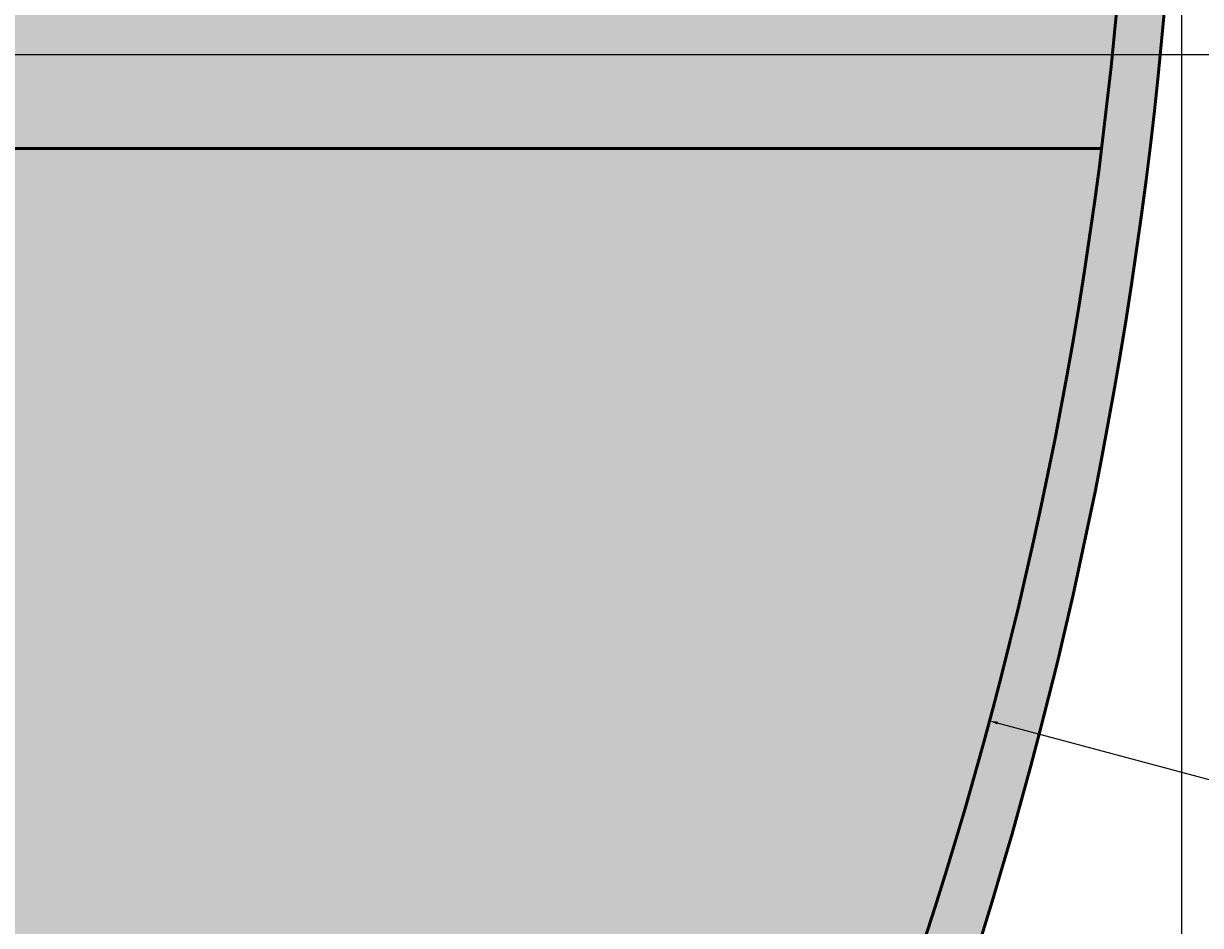
# Model space of a CAD drawing. Units: inches. Extents: x -12 to 334, y -10 to 186.
# Tile 71 of 77: x 257 to 282, y 64 to 83. Entities that reach past the tile are written whole.
import ezdxf

# ---------------------------------------------------------------- set-up
doc = ezdxf.new("R2010")
doc.units = ezdxf.units.IN
doc.header["$MEASUREMENT"] = 0
for name, color, linetype, lineweight in [('M-DIMS', 2, 'Continuous', 18), ('M-EQPM', 7, 'Continuous', 50), ('M-EQPM-PATT', 8, 'Continuous', 18)]:
    doc.layers.add(name, color=color, linetype=linetype, lineweight=lineweight)
doc.styles.get("Standard").update_dxf_attribs({"font": 'arial.ttf'})
doc.dimstyles.get("Standard").update_dxf_attribs({"dimtxt": 0.18, "dimasz": 0.18, "dimexe": 0.18, "dimexo": 0.0625, "dimgap": 0.09, "dimtad": 0, "dimtih": 1, "dimtoh": 1, "dimdec": 4, "dimzin": 0, "dimdsep": 46, "dimtxsty": 'Standard', "dimcen": 0.09, "dimadec": 0, "dimazin": 0, "dimtfac": 1, "dimtdec": 4, "dimtofl": 0, "dimtmove": 0, "dimatfit": 3, "dimfxl": 1, "dimtolj": 1, "dimtzin": 0, "dimarcsym": 0})

# ---------------------------------------------------------------- blocks, each defined once
blk = doc.blocks.new('*D1')
at = {"layer": 'Defpoints', "color": 0, "transparency": 16777216}
for p in [(281.426, 91.899), (3.376, 80.692), (281.426, 14.304)]:
    blk.add_point(p, dxfattribs=at)
at = {"layer": 'M-DIMS', "color": 0, "lineweight": -2, "transparency": 16777216}
for p, q in [((281.426, 91.836), (281.426, 14.124)), ((3.376, 80.629), (3.376, 14.124)), ((3.556, 14.304), (141.935, 14.304)), ((281.246, 14.304), (142.867, 14.304))]:
    blk.add_line(p, q, dxfattribs=at)
at = {"layer": 'M-DIMS', "color": 0, "transparency": 16777216}
for points in [[(3.556, 14.334), (3.556, 14.274), (3.376, 14.304)], [(281.246, 14.334), (281.246, 14.274), (281.426, 14.304)]]:
    blk.add_solid(points, dxfattribs=at)
at = {"layer": 'M-DIMS', "color": 0, "transparency": 16777216, "insert": (142.401, 14.304), "char_height": 0.18, "attachment_point": 5}
blk.add_mtext('\\A1;278.05', dxfattribs=at)
blk = doc.blocks.new('*D17')
at = {"layer": 'Defpoints', "color": 0, "transparency": 16777216}
for p in [(106.177, 102.896), (105.892, 56.321), (295.976, 56.321)]:
    blk.add_point(p, dxfattribs=at)
at = {"layer": 'M-DIMS', "color": 0, "lineweight": -2, "transparency": 16777216}
for p, q in [((106.24, 102.896), (296.156, 102.896)), ((295.976, 102.716), (295.976, 79.79)), ((295.976, 56.501), (295.976, 79.426)), ((105.954, 56.321), (296.156, 56.321))]:
    blk.add_line(p, q, dxfattribs=at)
at = {"layer": 'M-DIMS', "color": 0, "transparency": 16777216}
for points in [[(295.946, 102.716), (296.006, 102.716), (295.976, 102.896)], [(295.946, 56.501), (296.006, 56.501), (295.976, 56.321)]]:
    blk.add_solid(points, dxfattribs=at)
at = {"layer": 'M-DIMS', "color": 0, "transparency": 16777216, "insert": (295.976, 79.608), "char_height": 0.18, "attachment_point": 5}
blk.add_mtext('\\A1;46.575', dxfattribs=at)
blk = doc.blocks.new('*D24')
at = {"layer": 'Defpoints', "color": 0, "transparency": 16777216}
for p in [(269.381, 137.943), (269.381, 45.854), (295.976, 45.854)]:
    blk.add_point(p, dxfattribs=at)
at = {"layer": 'M-DIMS', "color": 0, "lineweight": -2, "transparency": 16777216}
for p, q in [((269.443, 137.943), (296.156, 137.943)), ((295.976, 137.763), (295.976, 92.081)), ((295.976, 46.034), (295.976, 91.717)), ((269.443, 45.854), (296.156, 45.854))]:
    blk.add_line(p, q, dxfattribs=at)
at = {"layer": 'M-DIMS', "color": 0, "transparency": 16777216}
for points in [[(295.946, 137.763), (296.006, 137.763), (295.976, 137.943)], [(295.946, 46.034), (296.006, 46.034), (295.976, 45.854)]]:
    blk.add_solid(points, dxfattribs=at)
at = {"layer": 'M-DIMS', "color": 0, "transparency": 16777216, "insert": (295.976, 91.899), "char_height": 0.18, "attachment_point": 5}
blk.add_mtext('\\A1;92.09', dxfattribs=at)
blk = doc.blocks.new('*D38')
at = {"layer": 'Defpoints', "color": 0, "transparency": 16777216}
for p in [(247.935, 82.697), (247.935, 46.854), (295.976, 46.854)]:
    blk.add_point(p, dxfattribs=at)
at = {"layer": 'M-DIMS', "color": 0, "lineweight": -2, "transparency": 16777216}
for p, q in [((247.998, 82.697), (296.156, 82.697)), ((295.976, 82.517), (295.976, 64.957)), ((295.976, 47.034), (295.976, 64.594)), ((247.998, 46.854), (296.156, 46.854))]:
    blk.add_line(p, q, dxfattribs=at)
at = {"layer": 'M-DIMS', "color": 0, "transparency": 16777216}
for points in [[(295.946, 82.517), (296.006, 82.517), (295.976, 82.697)], [(295.946, 47.034), (296.006, 47.034), (295.976, 46.854)]]:
    blk.add_solid(points, dxfattribs=at)
at = {"layer": 'M-DIMS', "color": 0, "transparency": 16777216, "insert": (295.976, 64.775), "char_height": 0.18, "attachment_point": 5}
blk.add_mtext('\\A1;35.84', dxfattribs=at)
blk = doc.blocks.new('*D39')
at = {"layer": 'Defpoints', "color": 0, "transparency": 16777216}
for p in [(279.726, 80.692), (-11.174, 45.854), (269.381, 45.854)]:
    blk.add_point(p, dxfattribs=at)
at = {"layer": 'M-DIMS', "color": 0, "lineweight": -2, "transparency": 16777216}
for p, q in [((279.664, 80.692), (-11.354, 80.692)), ((-11.174, 80.512), (-11.174, 63.455)), ((-11.174, 46.034), (-11.174, 63.091)), ((269.318, 45.854), (-11.354, 45.854))]:
    blk.add_line(p, q, dxfattribs=at)
at = {"layer": 'M-DIMS', "color": 0, "transparency": 16777216}
for points in [[(-11.204, 80.512), (-11.144, 80.512), (-11.174, 80.692)], [(-11.204, 46.034), (-11.144, 46.034), (-11.174, 45.854)]]:
    blk.add_solid(points, dxfattribs=at)
at = {"layer": 'M-DIMS', "color": 0, "transparency": 16777216, "insert": (-11.174, 63.273), "char_height": 0.18, "attachment_point": 5}
blk.add_mtext('\\A1;34.84', dxfattribs=at)
blk = doc.blocks.new('*D41')
at = {"layer": 'Defpoints', "color": 0, "transparency": 16777216}
for p in [(190.169, 91.899), (277.343, 68.515)]:
    blk.add_point(p, dxfattribs=at)
at = {"layer": 'M-DIMS', "color": 0, "lineweight": -2, "transparency": 16777216}
for p, q in [((190.079, 91.899), (190.259, 91.899)), ((190.169, 91.809), (190.169, 91.989)), ((329.648, 54.485), (277.517, 68.469)), ((329.828, 54.485), (329.648, 54.485))]:
    blk.add_line(p, q, dxfattribs=at)
at = {"layer": 'M-DIMS', "color": 0, "transparency": 16777216}
blk.add_solid([(277.525, 68.498), (277.509, 68.44), (277.343, 68.515)], dxfattribs=at)
at = {"layer": 'M-DIMS', "color": 0, "transparency": 16777216, "insert": (330.307, 54.485), "char_height": 0.18, "attachment_point": 5}
blk.add_mtext('\\A1;R90.26', dxfattribs=at)

msp = doc.modelspace()

# ---------------------------------------------------------------- hatches: boundary and pattern name
at = {"layer": 'M-EQPM-PATT', "transparency": 33554556}
h = msp.add_hatch(color=256, dxfattribs=at)
h.set_gradient(color1=(248, 206, 179), color2=(248, 206, 179), tint=1)
h.paths.add_polyline_path([(179.7818, 136.8871), (126.9567, 136.8871), (106.1771, 100.8958), (171.5458, 100.8958)])
h.paths.add_polyline_path([(268.3808, 136.9435), (214.0166, 136.9435), (214.0166, 154.8345), (196.3421, 154.8345), (196.3421, 136.8871), (179.7818, 136.8871), (171.5458, 100.8958), (231.7758, 100.8958, -0.4142136), (251.9801, 80.6915), (279.7263, 80.6915, 0.1631825)])
at = {"layer": 'M-EQPM-PATT'}
h = msp.add_hatch(color=256, dxfattribs=at)
h.set_gradient(color1=(99, 100, 102), color2=(99, 100, 102), tint=1)
h.paths.add_polyline_path([(126.9567, 136.8871), (179.7818, 136.8871), (180.0106, 137.8871), (126.3793, 137.8871), (106.1771, 102.8958), (86.8879, 102.8958), (86.8879, 109.0583), (84.7229, 109.0583), (84.7229, 100.8958), (106.1771, 100.8958)])
h.paths.add_polyline_path([(196.3421, 152.8345), (195.3421, 152.8345), (195.3421, 137.8871), (180.0106, 137.8871), (179.7818, 136.8871), (196.3421, 136.8871)])
h.paths.add_polyline_path([(215.0166, 152.8345), (214.0166, 152.8345), (214.0166, 136.9435), (268.3808, 136.9435, -0.2673785), (268.3808, 46.8541), (249.3759, 46.8541), (249.8485, 45.8541), (269.3808, 45.8541, 0.2615891), (269.3808, 137.9435), (215.0166, 137.9435)])
h = msp.add_hatch(color=256, dxfattribs=at)
h.set_gradient(color1=(94, 103, 175), color2=(94, 103, 175), tint=1)
h.paths.add_polyline_path([(129.093, 89.8963), (86.8879, 89.8963), (86.8879, 69.6117), (129.093, 69.6117)], flags=17)
h.paths.add_polyline_path([(170.9079, 89.8963), (130.8573, 89.8963), (130.8573, 69.6117), (170.9079, 69.6117)], flags=17)
h.paths.add_polyline_path([(216.4278, 89.8963), (172.6722, 89.8963), (172.6722, 69.6117), (216.4278, 69.6117)], flags=17)
h.paths.add_polyline_path([(245.9354, 82.6969), (247.9354, 82.6969), (247.9354, 46.8541), (268.3808, 46.8541, 0.0998398), (279.7263, 80.6915), (251.9801, 80.6915, 0.4142136), (231.7758, 100.8958), (84.7229, 100.8958), (84.7229, 109.0583), (83.7229, 109.0583), (83.7229, 95.8963), (129.093, 95.8963), (129.093, 98.1081), (130.8573, 98.1081), (130.8573, 95.8963), (170.9079, 95.8963), (170.9079, 98.1081), (172.6722, 98.1081), (172.6722, 95.8963), (216.4278, 95.8963), (216.4278, 98.1081), (218.1922, 98.1081), (218.1922, 95.8963), (226.6083, 95.8963, -1), (226.6083, 63.6117), (218.1922, 63.6117), (218.1922, 61.1045), (216.4278, 61.1045), (216.4278, 63.6117), (172.6722, 63.6117), (172.6722, 61.1045), (170.9079, 61.1045), (170.9079, 63.6117), (130.8573, 63.6117), (130.8573, 61.1045), (129.093, 61.1045), (129.093, 63.6117), (87.8879, 63.6117), (87.8879, 56.3205), (105.8919, 56.3205), (105.8919, 28.8541), (115.8919, 28.8541), (115.8919, 46.8541), (222.5761, 46.8541), (222.5761, 30.8541), (232.5761, 30.8541), (232.5761, 46.8541), (245.9354, 46.8541)])
h.paths.add_polyline_path([(86.8879, 89.8963), (75.9244, 89.8963), (75.9244, 69.6117), (86.8879, 69.6117)])
h.paths.add_polyline_path([(83.7229, 109.0583), (75.9244, 109.0583), (75.9244, 95.8963), (83.7229, 95.8963)])
h.paths.add_polyline_path([(226.6083, 89.8963), (218.1922, 89.8963), (218.1922, 69.6117), (226.6083, 69.6117, 1)], flags=17)
h = msp.add_hatch(color=256, dxfattribs=at)
h.set_gradient(color1=(0, 0, 255), color2=(0, 0, 255), tint=1)
h.paths.add_polyline_path([(84.7229, 100.8958), (84.7229, 109.0583), (83.7229, 109.0583), (83.7229, 95.8963), (129.093, 95.8963), (129.093, 98.1081), (130.8573, 98.1081), (130.8573, 95.8963), (170.9079, 95.8963), (170.9079, 98.1081), (172.6722, 98.1081), (172.6722, 95.8963), (216.4278, 95.8963), (216.4278, 98.1081), (218.1922, 98.1081), (218.1922, 95.8963), (226.6083, 95.8963, -1), (226.6083, 63.6117), (218.1922, 63.6117), (218.1922, 61.1045), (216.4278, 61.1045), (216.4278, 63.6117), (172.6722, 63.6117), (172.6722, 61.1045), (170.9079, 61.1045), (170.9079, 63.6117), (130.8573, 63.6117), (130.8573, 61.1045), (129.093, 61.1045), (129.093, 63.6117), (87.8879, 63.6117), (87.8879, 56.3205), (105.8919, 56.3205), (105.8919, 28.8541), (115.8919, 28.8541), (115.8919, 46.8541), (222.5761, 46.8541), (222.5761, 30.8541), (232.5761, 30.8541), (232.5761, 46.8541), (245.9354, 46.8541), (245.9354, 82.6969), (247.9354, 82.6969), (247.9354, 46.8541), (268.3808, 46.8541, 0.0998398), (279.7263, 80.6915), (251.9801, 80.6915, 0.4142136), (231.7758, 100.8958)])

# ---------------------------------------------------------------- linework, layer by layer
at = {"layer": 'M-EQPM'}
msp.add_line((251.9801, 80.6915), (279.7263, 80.6915), dxfattribs=at)
for centre, radius, start, end in [((187.3936, 91.8988), 94.032, 330.681071, 29.318929), ((190.1689, 91.8988), 90.256, 330.061028, 29.938972)]:
    msp.add_arc(centre, radius, start, end, dxfattribs=at)

# ---------------------------------------------------------------- dimensions: what is measured, and where the dimension line sits
at = {"layer": 'M-DIMS'}
for base, p1, p2, override, picture, middle in [((295.9756, 45.8541), (269.3808, 137.9435), (269.3808, 45.8541), {"dimdec": 2, "dimlfac": 1, "dimrnd": 0, "dimzin": 0, "dimdsep": 46, "dimlunit": 2}, '*D24', (295.9756, 91.8988)), ((295.9756, 56.3205), (106.1771, 102.8958), (105.8919, 56.3205), {"dimdec": 3, "dimlfac": 1, "dimrnd": 0, "dimzin": 0, "dimdsep": 46, "dimlunit": 2}, '*D17', (295.9756, 79.6082)), ((295.9756, 46.8541), (247.9354, 82.6969), (247.9354, 46.8541), {"dimdec": 2, "dimlfac": 1, "dimrnd": 0, "dimzin": 0, "dimdsep": 46, "dimlunit": 2}, '*D38', (295.9756, 64.7755)), ((-11.1736, 45.8541), (279.7263, 80.6915), (269.3808, 45.8541), {"dimdec": 2, "dimlfac": 1, "dimrnd": 0, "dimzin": 0, "dimdsep": 46, "dimlunit": 2}, '*D39', (-11.1735, 63.2728))]:
    dim = msp.add_linear_dim(base=base, p1=p1, p2=p2, angle=90, dimstyle='Standard', override=override, dxfattribs=at)
    dim.commit()
    dim.dimension.update_dxf_attribs({"geometry": picture, "text_midpoint": middle})
dim = msp.add_linear_dim(base=(281.4256, 14.3041), p1=(3.3765, 80.6915), p2=(281.4256, 91.8988), dimstyle='Standard', override={"dimdec": 2, "dimlfac": 1, "dimrnd": 0, "dimzin": 0, "dimdsep": 46, "dimlunit": 2}, dxfattribs=at)
dim.commit()
dim.dimension.update_dxf_attribs({"geometry": '*D1', "text_midpoint": (142.401, 14.3041)})
dim = msp.add_radius_dim(center=(190.1689, 91.8988), mpoint=(277.3431, 68.5153), dimstyle='Standard', override={"dimdec": 2, "dimlfac": 1, "dimrnd": 0, "dimzin": 0, "dimdsep": 46, "dimlunit": 2}, dxfattribs=at)
dim.commit()
dim.dimension.update_dxf_attribs({"geometry": '*D41', "text_midpoint": (330.3074, 54.4851), "dimtype": 164})

doc.saveas('drawing.dxf')
